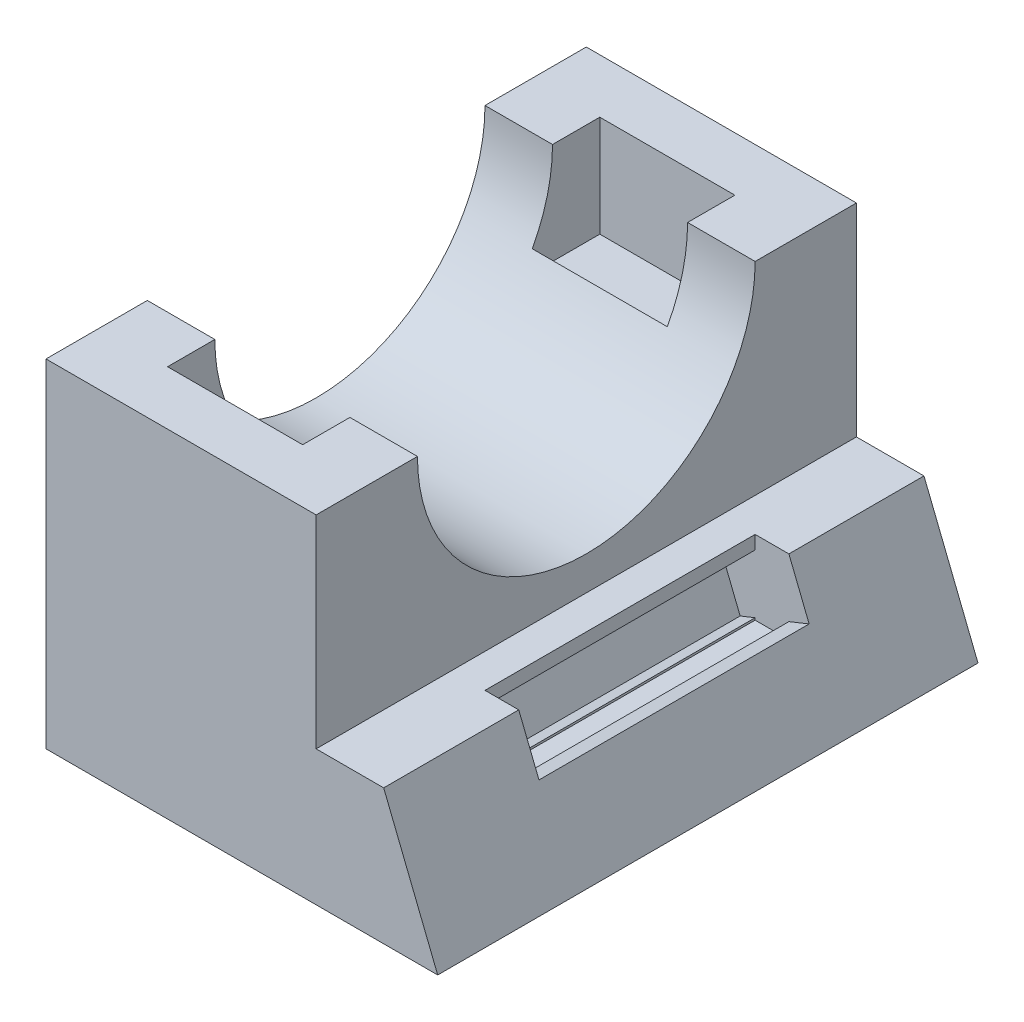
ISO-10303-21;
HEADER;
FILE_DESCRIPTION(('STEP AP214'),'2;1');
FILE_NAME('part.step','',(''),(''),'','','');
FILE_SCHEMA(('AUTOMOTIVE_DESIGN { 1 0 10303 214 1 1 1 1 }'));
ENDSEC;
DATA;
#1=APPLICATION_CONTEXT('core data for automotive mechanical design processes');
#2=APPLICATION_PROTOCOL_DEFINITION('international standard','automotive_design',2000,#1);
#3=PRODUCT_CONTEXT('',#1,'mechanical');
#4=PRODUCT('Part','Part','',(#3));
#5=PRODUCT_RELATED_PRODUCT_CATEGORY('part','',(#4));
#6=PRODUCT_DEFINITION_FORMATION('','',#4);
#7=PRODUCT_DEFINITION_CONTEXT('part definition',#1,'design');
#8=PRODUCT_DEFINITION('design','',#6,#7);
#9=PRODUCT_DEFINITION_SHAPE('','',#8);
#10=(LENGTH_UNIT() NAMED_UNIT(*) SI_UNIT(.MILLI.,.METRE.));
#11=(NAMED_UNIT(*) PLANE_ANGLE_UNIT() SI_UNIT($,.RADIAN.));
#12=(NAMED_UNIT(*) SI_UNIT($,.STERADIAN.) SOLID_ANGLE_UNIT());
#13=UNCERTAINTY_MEASURE_WITH_UNIT(LENGTH_MEASURE(1.E-05),#10,'distance_accuracy_value','');
#14=(GEOMETRIC_REPRESENTATION_CONTEXT(3) GLOBAL_UNCERTAINTY_ASSIGNED_CONTEXT((#13)) GLOBAL_UNIT_ASSIGNED_CONTEXT((#10,
#11,#12)) REPRESENTATION_CONTEXT('',''));
#15=CARTESIAN_POINT('',(0.,0.,0.));
#16=DIRECTION('',(0.,0.,1.));
#17=DIRECTION('',(1.,0.,0.));
#18=AXIS2_PLACEMENT_3D('',#15,#16,#17);
#19=CARTESIAN_POINT('',(45.,9.00000000000001,20.));
#20=DIRECTION('',(-1.,0.,0.));
#21=DIRECTION('',(0.,0.,1.));
#22=AXIS2_PLACEMENT_3D('',#19,#20,#21);
#23=PLANE('',#22);
#24=DIRECTION('',(0.,1.,0.));
#25=VECTOR('',#24,1.);
#26=CARTESIAN_POINT('',(45.,9.00000000000001,60.));
#27=LINE('',#26,#25);
#28=CARTESIAN_POINT('',(45.,18.,60.));
#29=VERTEX_POINT('',#28);
#30=CARTESIAN_POINT('',(45.,20.,60.));
#31=VERTEX_POINT('',#30);
#32=EDGE_CURVE('E297',#29,#31,#27,.T.);
#33=ORIENTED_EDGE('',*,*,#32,.F.);
#34=DIRECTION('',(0.,0.,-1.));
#35=VECTOR('',#34,1.);
#36=CARTESIAN_POINT('',(45.,18.,20.));
#37=LINE('',#36,#35);
#38=CARTESIAN_POINT('',(45.,18.,20.));
#39=VERTEX_POINT('',#38);
#40=EDGE_CURVE('E229',#29,#39,#37,.T.);
#41=ORIENTED_EDGE('',*,*,#40,.T.);
#42=DIRECTION('',(0.,1.,0.));
#43=VECTOR('',#42,1.);
#44=CARTESIAN_POINT('',(45.,9.00000000000001,20.));
#45=LINE('',#44,#43);
#46=CARTESIAN_POINT('',(45.,20.,20.));
#47=VERTEX_POINT('',#46);
#48=EDGE_CURVE('E298',#39,#47,#45,.T.);
#49=ORIENTED_EDGE('',*,*,#48,.T.);
#50=DIRECTION('',(0.,0.,1.));
#51=VECTOR('',#50,1.);
#52=CARTESIAN_POINT('',(45.,20.,20.));
#53=LINE('',#52,#51);
#54=EDGE_CURVE('E283',#47,#31,#53,.T.);
#55=ORIENTED_EDGE('',*,*,#54,.T.);
#56=EDGE_LOOP('',(#33,#41,#49,#55));
#57=FACE_BOUND('',#56,.T.);
#58=ADVANCED_FACE('F39',(#57),#23,.F.);
#59=CARTESIAN_POINT('',(0.,50.,80.));
#60=DIRECTION('',(0.,-1.,0.));
#61=DIRECTION('',(0.,0.,-1.));
#62=AXIS2_PLACEMENT_3D('',#59,#60,#61);
#63=PLANE('',#62);
#64=DIRECTION('',(0.,0.,-1.));
#65=VECTOR('',#64,1.);
#66=CARTESIAN_POINT('',(0.,50.,80.));
#67=LINE('',#66,#65);
#68=CARTESIAN_POINT('',(0.,50.,15.));
#69=VERTEX_POINT('',#68);
#70=CARTESIAN_POINT('',(0.,50.,0.));
#71=VERTEX_POINT('',#70);
#72=EDGE_CURVE('E428',#69,#71,#67,.T.);
#73=ORIENTED_EDGE('',*,*,#72,.F.);
#74=DIRECTION('',(1.,0.,0.));
#75=VECTOR('',#74,1.);
#76=CARTESIAN_POINT('',(0.,50.,15.));
#77=LINE('',#76,#75);
#78=CARTESIAN_POINT('',(10.,50.,15.));
#79=VERTEX_POINT('',#78);
#80=EDGE_CURVE('E323',#69,#79,#77,.T.);
#81=ORIENTED_EDGE('',*,*,#80,.T.);
#82=DIRECTION('',(0.,0.,1.));
#83=VECTOR('',#82,1.);
#84=CARTESIAN_POINT('',(10.,50.,18.));
#85=LINE('',#84,#83);
#86=CARTESIAN_POINT('',(10.,50.,8.00000000000001));
#87=VERTEX_POINT('',#86);
#88=EDGE_CURVE('E341',#87,#79,#85,.T.);
#89=ORIENTED_EDGE('',*,*,#88,.F.);
#90=DIRECTION('',(-1.,0.,0.));
#91=VECTOR('',#90,1.);
#92=CARTESIAN_POINT('',(10.,50.,8.00000000000001));
#93=LINE('',#92,#91);
#94=CARTESIAN_POINT('',(30.,50.,8.00000000000001));
#95=VERTEX_POINT('',#94);
#96=EDGE_CURVE('E353',#95,#87,#93,.T.);
#97=ORIENTED_EDGE('',*,*,#96,.F.);
#98=DIRECTION('',(0.,0.,-1.));
#99=VECTOR('',#98,1.);
#100=CARTESIAN_POINT('',(30.,50.,8.00000000000001));
#101=LINE('',#100,#99);
#102=CARTESIAN_POINT('',(30.,50.,15.));
#103=VERTEX_POINT('',#102);
#104=EDGE_CURVE('E355',#103,#95,#101,.T.);
#105=ORIENTED_EDGE('',*,*,#104,.F.);
#106=CARTESIAN_POINT('',(40.,50.,15.));
#107=VERTEX_POINT('',#106);
#108=EDGE_CURVE('E317',#103,#107,#77,.T.);
#109=ORIENTED_EDGE('',*,*,#108,.T.);
#110=DIRECTION('',(0.,0.,-1.));
#111=VECTOR('',#110,1.);
#112=CARTESIAN_POINT('',(40.,50.,80.));
#113=LINE('',#112,#111);
#114=CARTESIAN_POINT('',(40.,50.,0.));
#115=VERTEX_POINT('',#114);
#116=EDGE_CURVE('E435',#107,#115,#113,.T.);
#117=ORIENTED_EDGE('',*,*,#116,.T.);
#118=DIRECTION('',(-1.,0.,0.));
#119=VECTOR('',#118,1.);
#120=CARTESIAN_POINT('',(0.,50.,0.));
#121=LINE('',#120,#119);
#122=EDGE_CURVE('E425',#115,#71,#121,.T.);
#123=ORIENTED_EDGE('',*,*,#122,.T.);
#124=EDGE_LOOP('',(#73,#81,#89,#97,#105,#109,#117,#123));
#125=FACE_BOUND('',#124,.T.);
#126=ADVANCED_FACE('F456',(#125),#63,.F.);
#127=CARTESIAN_POINT('',(58.,0.,80.));
#128=DIRECTION('',(0.,1.,0.));
#129=DIRECTION('',(0.,0.,1.));
#130=AXIS2_PLACEMENT_3D('',#127,#128,#129);
#131=PLANE('',#130);
#132=DIRECTION('',(1.,0.,0.));
#133=VECTOR('',#132,1.);
#134=CARTESIAN_POINT('',(58.,0.,0.));
#135=LINE('',#134,#133);
#136=CARTESIAN_POINT('',(0.,0.,0.));
#137=VERTEX_POINT('',#136);
#138=CARTESIAN_POINT('',(58.,0.,0.));
#139=VERTEX_POINT('',#138);
#140=EDGE_CURVE('E365',#137,#139,#135,.T.);
#141=ORIENTED_EDGE('',*,*,#140,.T.);
#142=DIRECTION('',(0.,0.,-1.));
#143=VECTOR('',#142,1.);
#144=CARTESIAN_POINT('',(58.,0.,80.));
#145=LINE('',#144,#143);
#146=CARTESIAN_POINT('',(58.,0.,80.));
#147=VERTEX_POINT('',#146);
#148=EDGE_CURVE('E50',#147,#139,#145,.T.);
#149=ORIENTED_EDGE('',*,*,#148,.F.);
#150=DIRECTION('',(1.,0.,0.));
#151=VECTOR('',#150,1.);
#152=CARTESIAN_POINT('',(58.,0.,80.));
#153=LINE('',#152,#151);
#154=CARTESIAN_POINT('',(0.,0.,80.));
#155=VERTEX_POINT('',#154);
#156=EDGE_CURVE('E405',#155,#147,#153,.T.);
#157=ORIENTED_EDGE('',*,*,#156,.F.);
#158=DIRECTION('',(0.,0.,-1.));
#159=VECTOR('',#158,1.);
#160=CARTESIAN_POINT('',(0.,0.,80.));
#161=LINE('',#160,#159);
#162=EDGE_CURVE('E414',#155,#137,#161,.T.);
#163=ORIENTED_EDGE('',*,*,#162,.T.);
#164=EDGE_LOOP('',(#141,#149,#157,#163));
#165=FACE_BOUND('',#164,.T.);
#166=ADVANCED_FACE('F41',(#165),#131,.F.);
#167=CARTESIAN_POINT('',(40.,20.,80.));
#168=DIRECTION('',(0.,-1.,0.));
#169=DIRECTION('',(0.,0.,-1.));
#170=AXIS2_PLACEMENT_3D('',#167,#168,#169);
#171=PLANE('',#170);
#172=DIRECTION('',(0.,0.,1.));
#173=VECTOR('',#172,1.);
#174=CARTESIAN_POINT('',(50.,20.,0.));
#175=LINE('',#174,#173);
#176=CARTESIAN_POINT('',(50.,20.,60.));
#177=VERTEX_POINT('',#176);
#178=CARTESIAN_POINT('',(50.,20.,80.));
#179=VERTEX_POINT('',#178);
#180=EDGE_CURVE('E308',#177,#179,#175,.T.);
#181=ORIENTED_EDGE('',*,*,#180,.F.);
#182=DIRECTION('',(1.,0.,0.));
#183=VECTOR('',#182,1.);
#184=CARTESIAN_POINT('',(45.,20.,60.));
#185=LINE('',#184,#183);
#186=EDGE_CURVE('E272',#31,#177,#185,.T.);
#187=ORIENTED_EDGE('',*,*,#186,.F.);
#188=ORIENTED_EDGE('',*,*,#54,.F.);
#189=DIRECTION('',(-1.,0.,0.));
#190=VECTOR('',#189,1.);
#191=CARTESIAN_POINT('',(50.,20.,20.));
#192=LINE('',#191,#190);
#193=CARTESIAN_POINT('',(50.,20.,20.));
#194=VERTEX_POINT('',#193);
#195=EDGE_CURVE('E268',#194,#47,#192,.T.);
#196=ORIENTED_EDGE('',*,*,#195,.F.);
#197=CARTESIAN_POINT('',(50.,20.,0.));
#198=VERTEX_POINT('',#197);
#199=EDGE_CURVE('E306',#198,#194,#175,.T.);
#200=ORIENTED_EDGE('',*,*,#199,.F.);
#201=DIRECTION('',(-1.,0.,0.));
#202=VECTOR('',#201,1.);
#203=CARTESIAN_POINT('',(40.,20.,0.));
#204=LINE('',#203,#202);
#205=CARTESIAN_POINT('',(40.,20.,0.));
#206=VERTEX_POINT('',#205);
#207=EDGE_CURVE('E417',#198,#206,#204,.T.);
#208=ORIENTED_EDGE('',*,*,#207,.T.);
#209=DIRECTION('',(0.,0.,-1.));
#210=VECTOR('',#209,1.);
#211=CARTESIAN_POINT('',(40.,20.,80.));
#212=LINE('',#211,#210);
#213=CARTESIAN_POINT('',(40.,20.,80.));
#214=VERTEX_POINT('',#213);
#215=EDGE_CURVE('E436',#214,#206,#212,.T.);
#216=ORIENTED_EDGE('',*,*,#215,.F.);
#217=DIRECTION('',(-1.,0.,0.));
#218=VECTOR('',#217,1.);
#219=CARTESIAN_POINT('',(40.,20.,80.));
#220=LINE('',#219,#218);
#221=EDGE_CURVE('E403',#179,#214,#220,.T.);
#222=ORIENTED_EDGE('',*,*,#221,.F.);
#223=EDGE_LOOP('',(#181,#187,#188,#196,#200,#208,#216,#222));
#224=FACE_BOUND('',#223,.T.);
#225=ADVANCED_FACE('F473',(#224),#171,.F.);
#226=CARTESIAN_POINT('',(40.,50.,80.));
#227=DIRECTION('',(-1.,0.,0.));
#228=DIRECTION('',(0.,-1.,0.));
#229=AXIS2_PLACEMENT_3D('',#226,#227,#228);
#230=PLANE('',#229);
#231=ORIENTED_EDGE('',*,*,#116,.F.);
#232=CARTESIAN_POINT('',(40.,50.,40.));
#233=DIRECTION('',(1.,0.,0.));
#234=DIRECTION('',(0.,1.,0.));
#235=AXIS2_PLACEMENT_3D('',#232,#233,#234);
#236=CIRCLE('',#235,25.);
#237=CARTESIAN_POINT('',(40.,50.,65.));
#238=VERTEX_POINT('',#237);
#239=EDGE_CURVE('E313',#238,#107,#236,.T.);
#240=ORIENTED_EDGE('',*,*,#239,.F.);
#241=CARTESIAN_POINT('',(40.,50.,80.));
#242=VERTEX_POINT('',#241);
#243=EDGE_CURVE('E433',#242,#238,#113,.T.);
#244=ORIENTED_EDGE('',*,*,#243,.F.);
#245=DIRECTION('',(0.,1.,0.));
#246=VECTOR('',#245,1.);
#247=CARTESIAN_POINT('',(40.,50.,80.));
#248=LINE('',#247,#246);
#249=EDGE_CURVE('E410',#214,#242,#248,.T.);
#250=ORIENTED_EDGE('',*,*,#249,.F.);
#251=ORIENTED_EDGE('',*,*,#215,.T.);
#252=DIRECTION('',(0.,1.,0.));
#253=VECTOR('',#252,1.);
#254=CARTESIAN_POINT('',(40.,50.,0.));
#255=LINE('',#254,#253);
#256=EDGE_CURVE('E420',#206,#115,#255,.T.);
#257=ORIENTED_EDGE('',*,*,#256,.T.);
#258=EDGE_LOOP('',(#231,#240,#244,#250,#251,#257));
#259=FACE_BOUND('',#258,.T.);
#260=ADVANCED_FACE('F461',(#259),#230,.F.);
#261=ORIENTED_EDGE('',*,*,#243,.T.);
#262=DIRECTION('',(1.,0.,0.));
#263=VECTOR('',#262,1.);
#264=CARTESIAN_POINT('',(0.,50.,65.));
#265=LINE('',#264,#263);
#266=CARTESIAN_POINT('',(30.,50.,65.));
#267=VERTEX_POINT('',#266);
#268=EDGE_CURVE('E337',#238,#267,#265,.F.);
#269=ORIENTED_EDGE('',*,*,#268,.T.);
#270=DIRECTION('',(0.,0.,-1.));
#271=VECTOR('',#270,1.);
#272=CARTESIAN_POINT('',(30.,50.,72.));
#273=LINE('',#272,#271);
#274=CARTESIAN_POINT('',(30.,50.,72.));
#275=VERTEX_POINT('',#274);
#276=EDGE_CURVE('E376',#275,#267,#273,.T.);
#277=ORIENTED_EDGE('',*,*,#276,.F.);
#278=DIRECTION('',(1.,0.,0.));
#279=VECTOR('',#278,1.);
#280=CARTESIAN_POINT('',(10.,50.,72.));
#281=LINE('',#280,#279);
#282=CARTESIAN_POINT('',(10.,50.,72.));
#283=VERTEX_POINT('',#282);
#284=EDGE_CURVE('E389',#283,#275,#281,.T.);
#285=ORIENTED_EDGE('',*,*,#284,.F.);
#286=DIRECTION('',(0.,0.,1.));
#287=VECTOR('',#286,1.);
#288=CARTESIAN_POINT('',(10.,50.,62.));
#289=LINE('',#288,#287);
#290=CARTESIAN_POINT('',(10.,50.,65.));
#291=VERTEX_POINT('',#290);
#292=EDGE_CURVE('E387',#291,#283,#289,.T.);
#293=ORIENTED_EDGE('',*,*,#292,.F.);
#294=CARTESIAN_POINT('',(0.,50.,65.));
#295=VERTEX_POINT('',#294);
#296=EDGE_CURVE('E335',#291,#295,#265,.F.);
#297=ORIENTED_EDGE('',*,*,#296,.T.);
#298=CARTESIAN_POINT('',(0.,50.,80.));
#299=VERTEX_POINT('',#298);
#300=EDGE_CURVE('E427',#299,#295,#67,.T.);
#301=ORIENTED_EDGE('',*,*,#300,.F.);
#302=DIRECTION('',(-1.,0.,0.));
#303=VECTOR('',#302,1.);
#304=CARTESIAN_POINT('',(0.,50.,80.));
#305=LINE('',#304,#303);
#306=EDGE_CURVE('E408',#242,#299,#305,.T.);
#307=ORIENTED_EDGE('',*,*,#306,.F.);
#308=EDGE_LOOP('',(#261,#269,#277,#285,#293,#297,#301,#307));
#309=FACE_BOUND('',#308,.T.);
#310=ADVANCED_FACE('F488',(#309),#63,.F.);
#311=CARTESIAN_POINT('',(0.,0.,80.));
#312=DIRECTION('',(1.,0.,0.));
#313=DIRECTION('',(0.,0.,-1.));
#314=AXIS2_PLACEMENT_3D('',#311,#312,#313);
#315=PLANE('',#314);
#316=ORIENTED_EDGE('',*,*,#300,.T.);
#317=CARTESIAN_POINT('',(0.,50.,40.));
#318=DIRECTION('',(1.,0.,0.));
#319=DIRECTION('',(0.,1.,0.));
#320=AXIS2_PLACEMENT_3D('',#317,#318,#319);
#321=CIRCLE('',#320,25.);
#322=EDGE_CURVE('E315',#295,#69,#321,.T.);
#323=ORIENTED_EDGE('',*,*,#322,.T.);
#324=ORIENTED_EDGE('',*,*,#72,.T.);
#325=DIRECTION('',(0.,-1.,0.));
#326=VECTOR('',#325,1.);
#327=CARTESIAN_POINT('',(0.,0.,0.));
#328=LINE('',#327,#326);
#329=EDGE_CURVE('E407',#71,#137,#328,.T.);
#330=ORIENTED_EDGE('',*,*,#329,.T.);
#331=ORIENTED_EDGE('',*,*,#162,.F.);
#332=DIRECTION('',(0.,-1.,0.));
#333=VECTOR('',#332,1.);
#334=CARTESIAN_POINT('',(0.,0.,80.));
#335=LINE('',#334,#333);
#336=EDGE_CURVE('E415',#299,#155,#335,.T.);
#337=ORIENTED_EDGE('',*,*,#336,.F.);
#338=EDGE_LOOP('',(#316,#323,#324,#330,#331,#337));
#339=FACE_BOUND('',#338,.T.);
#340=ADVANCED_FACE('F454',(#339),#315,.F.);
#341=CARTESIAN_POINT('',(0.,0.,80.));
#342=DIRECTION('',(0.,0.,-1.));
#343=DIRECTION('',(-1.,0.,0.));
#344=AXIS2_PLACEMENT_3D('',#341,#342,#343);
#345=PLANE('',#344);
#346=ORIENTED_EDGE('',*,*,#156,.T.);
#347=DIRECTION('',(0.371390676354104,-0.928476690885259,0.));
#348=VECTOR('',#347,1.);
#349=CARTESIAN_POINT('',(58.,0.,80.));
#350=LINE('',#349,#348);
#351=EDGE_CURVE('E291',#179,#147,#350,.T.);
#352=ORIENTED_EDGE('',*,*,#351,.F.);
#353=ORIENTED_EDGE('',*,*,#221,.T.);
#354=ORIENTED_EDGE('',*,*,#249,.T.);
#355=ORIENTED_EDGE('',*,*,#306,.T.);
#356=ORIENTED_EDGE('',*,*,#336,.T.);
#357=EDGE_LOOP('',(#346,#352,#353,#354,#355,#356));
#358=FACE_BOUND('',#357,.T.);
#359=ADVANCED_FACE('F482',(#358),#345,.F.);
#360=CARTESIAN_POINT('',(0.,0.,0.));
#361=DIRECTION('',(0.,0.,-1.));
#362=DIRECTION('',(-1.,0.,0.));
#363=AXIS2_PLACEMENT_3D('',#360,#361,#362);
#364=PLANE('',#363);
#365=DIRECTION('',(0.371390676354104,-0.928476690885259,0.));
#366=VECTOR('',#365,1.);
#367=CARTESIAN_POINT('',(58.,0.,0.));
#368=LINE('',#367,#366);
#369=EDGE_CURVE('E301',#198,#139,#368,.T.);
#370=ORIENTED_EDGE('',*,*,#369,.T.);
#371=ORIENTED_EDGE('',*,*,#140,.F.);
#372=ORIENTED_EDGE('',*,*,#329,.F.);
#373=ORIENTED_EDGE('',*,*,#122,.F.);
#374=ORIENTED_EDGE('',*,*,#256,.F.);
#375=ORIENTED_EDGE('',*,*,#207,.F.);
#376=EDGE_LOOP('',(#370,#371,#372,#373,#374,#375));
#377=FACE_BOUND('',#376,.T.);
#378=ADVANCED_FACE('F450',(#377),#364,.T.);
#379=CARTESIAN_POINT('',(30.,35.,62.));
#380=DIRECTION('',(0.,0.,-1.));
#381=DIRECTION('',(-1.,0.,0.));
#382=AXIS2_PLACEMENT_3D('',#379,#380,#381);
#383=PLANE('',#382);
#384=DIRECTION('',(0.,1.,0.));
#385=VECTOR('',#384,1.);
#386=CARTESIAN_POINT('',(30.,35.,62.));
#387=LINE('',#386,#385);
#388=CARTESIAN_POINT('',(30.,35.,62.));
#389=VERTEX_POINT('',#388);
#390=CARTESIAN_POINT('',(30.,38.1256579129621,62.));
#391=VERTEX_POINT('',#390);
#392=EDGE_CURVE('E358',#389,#391,#387,.T.);
#393=ORIENTED_EDGE('',*,*,#392,.T.);
#394=DIRECTION('',(1.,0.,0.));
#395=VECTOR('',#394,1.);
#396=CARTESIAN_POINT('',(0.,38.1256579129621,62.));
#397=LINE('',#396,#395);
#398=CARTESIAN_POINT('',(10.,38.1256579129621,62.));
#399=VERTEX_POINT('',#398);
#400=EDGE_CURVE('E328',#391,#399,#397,.F.);
#401=ORIENTED_EDGE('',*,*,#400,.T.);
#402=DIRECTION('',(0.,1.,0.));
#403=VECTOR('',#402,1.);
#404=CARTESIAN_POINT('',(10.,35.,62.));
#405=LINE('',#404,#403);
#406=CARTESIAN_POINT('',(10.,35.,62.));
#407=VERTEX_POINT('',#406);
#408=EDGE_CURVE('E384',#407,#399,#405,.T.);
#409=ORIENTED_EDGE('',*,*,#408,.F.);
#410=DIRECTION('',(-1.,0.,0.));
#411=VECTOR('',#410,1.);
#412=CARTESIAN_POINT('',(30.,35.,62.));
#413=LINE('',#412,#411);
#414=EDGE_CURVE('E375',#389,#407,#413,.T.);
#415=ORIENTED_EDGE('',*,*,#414,.F.);
#416=EDGE_LOOP('',(#393,#401,#409,#415));
#417=FACE_BOUND('',#416,.T.);
#418=ADVANCED_FACE('F604',(#417),#383,.F.);
#419=CARTESIAN_POINT('',(30.,35.,72.));
#420=DIRECTION('',(1.,0.,0.));
#421=DIRECTION('',(0.,0.,-1.));
#422=AXIS2_PLACEMENT_3D('',#419,#420,#421);
#423=PLANE('',#422);
#424=ORIENTED_EDGE('',*,*,#276,.T.);
#425=CARTESIAN_POINT('',(30.,50.,40.));
#426=DIRECTION('',(1.,0.,0.));
#427=DIRECTION('',(0.,0.,-1.));
#428=AXIS2_PLACEMENT_3D('',#425,#426,#427);
#429=CIRCLE('',#428,25.);
#430=EDGE_CURVE('E333',#267,#391,#429,.T.);
#431=ORIENTED_EDGE('',*,*,#430,.T.);
#432=ORIENTED_EDGE('',*,*,#392,.F.);
#433=DIRECTION('',(0.,0.,-1.));
#434=VECTOR('',#433,1.);
#435=CARTESIAN_POINT('',(30.,35.,72.));
#436=LINE('',#435,#434);
#437=CARTESIAN_POINT('',(30.,35.,72.));
#438=VERTEX_POINT('',#437);
#439=EDGE_CURVE('E385',#438,#389,#436,.T.);
#440=ORIENTED_EDGE('',*,*,#439,.F.);
#441=DIRECTION('',(0.,1.,0.));
#442=VECTOR('',#441,1.);
#443=CARTESIAN_POINT('',(30.,35.,72.));
#444=LINE('',#443,#442);
#445=EDGE_CURVE('E393',#438,#275,#444,.T.);
#446=ORIENTED_EDGE('',*,*,#445,.T.);
#447=EDGE_LOOP('',(#424,#431,#432,#440,#446));
#448=FACE_BOUND('',#447,.T.);
#449=ADVANCED_FACE('F663',(#448),#423,.F.);
#450=CARTESIAN_POINT('',(10.,35.,72.));
#451=DIRECTION('',(0.,0.,1.));
#452=DIRECTION('',(1.,0.,0.));
#453=AXIS2_PLACEMENT_3D('',#450,#451,#452);
#454=PLANE('',#453);
#455=ORIENTED_EDGE('',*,*,#284,.T.);
#456=ORIENTED_EDGE('',*,*,#445,.F.);
#457=DIRECTION('',(1.,0.,0.));
#458=VECTOR('',#457,1.);
#459=CARTESIAN_POINT('',(10.,35.,72.));
#460=LINE('',#459,#458);
#461=CARTESIAN_POINT('',(10.,35.,72.));
#462=VERTEX_POINT('',#461);
#463=EDGE_CURVE('E377',#462,#438,#460,.T.);
#464=ORIENTED_EDGE('',*,*,#463,.F.);
#465=DIRECTION('',(0.,1.,0.));
#466=VECTOR('',#465,1.);
#467=CARTESIAN_POINT('',(10.,35.,72.));
#468=LINE('',#467,#466);
#469=EDGE_CURVE('E400',#462,#283,#468,.T.);
#470=ORIENTED_EDGE('',*,*,#469,.T.);
#471=EDGE_LOOP('',(#455,#456,#464,#470));
#472=FACE_BOUND('',#471,.T.);
#473=ADVANCED_FACE('F657',(#472),#454,.F.);
#474=CARTESIAN_POINT('',(10.,35.,62.));
#475=DIRECTION('',(-1.,0.,0.));
#476=DIRECTION('',(0.,0.,1.));
#477=AXIS2_PLACEMENT_3D('',#474,#475,#476);
#478=PLANE('',#477);
#479=ORIENTED_EDGE('',*,*,#408,.T.);
#480=CARTESIAN_POINT('',(9.99999999999999,50.,40.));
#481=DIRECTION('',(-1.,0.,0.));
#482=DIRECTION('',(0.,0.,1.));
#483=AXIS2_PLACEMENT_3D('',#480,#481,#482);
#484=CIRCLE('',#483,25.);
#485=EDGE_CURVE('E326',#399,#291,#484,.T.);
#486=ORIENTED_EDGE('',*,*,#485,.T.);
#487=ORIENTED_EDGE('',*,*,#292,.T.);
#488=ORIENTED_EDGE('',*,*,#469,.F.);
#489=DIRECTION('',(0.,0.,1.));
#490=VECTOR('',#489,1.);
#491=CARTESIAN_POINT('',(10.,35.,62.));
#492=LINE('',#491,#490);
#493=EDGE_CURVE('E374',#407,#462,#492,.T.);
#494=ORIENTED_EDGE('',*,*,#493,.F.);
#495=EDGE_LOOP('',(#479,#486,#487,#488,#494));
#496=FACE_BOUND('',#495,.T.);
#497=ADVANCED_FACE('F652',(#496),#478,.F.);
#498=CARTESIAN_POINT('',(0.,35.,0.));
#499=DIRECTION('',(0.,1.,0.));
#500=DIRECTION('',(0.,0.,1.));
#501=AXIS2_PLACEMENT_3D('',#498,#499,#500);
#502=PLANE('',#501);
#503=ORIENTED_EDGE('',*,*,#414,.T.);
#504=ORIENTED_EDGE('',*,*,#493,.T.);
#505=ORIENTED_EDGE('',*,*,#463,.T.);
#506=ORIENTED_EDGE('',*,*,#439,.T.);
#507=EDGE_LOOP('',(#503,#504,#505,#506));
#508=FACE_BOUND('',#507,.T.);
#509=ADVANCED_FACE('F648',(#508),#502,.T.);
#510=CARTESIAN_POINT('',(30.,35.,18.));
#511=DIRECTION('',(0.,0.,1.));
#512=DIRECTION('',(1.,0.,0.));
#513=AXIS2_PLACEMENT_3D('',#510,#511,#512);
#514=PLANE('',#513);
#515=DIRECTION('',(0.,1.,0.));
#516=VECTOR('',#515,1.);
#517=CARTESIAN_POINT('',(10.,35.,18.));
#518=LINE('',#517,#516);
#519=CARTESIAN_POINT('',(10.,35.,18.));
#520=VERTEX_POINT('',#519);
#521=CARTESIAN_POINT('',(10.,38.1256579129621,18.));
#522=VERTEX_POINT('',#521);
#523=EDGE_CURVE('E363',#520,#522,#518,.T.);
#524=ORIENTED_EDGE('',*,*,#523,.T.);
#525=DIRECTION('',(1.,0.,0.));
#526=VECTOR('',#525,1.);
#527=CARTESIAN_POINT('',(0.,38.125657912962,18.));
#528=LINE('',#527,#526);
#529=CARTESIAN_POINT('',(30.,38.1256579129621,18.));
#530=VERTEX_POINT('',#529);
#531=EDGE_CURVE('E312',#522,#530,#528,.T.);
#532=ORIENTED_EDGE('',*,*,#531,.T.);
#533=DIRECTION('',(0.,1.,0.));
#534=VECTOR('',#533,1.);
#535=CARTESIAN_POINT('',(30.,35.,18.));
#536=LINE('',#535,#534);
#537=CARTESIAN_POINT('',(30.,35.,18.));
#538=VERTEX_POINT('',#537);
#539=EDGE_CURVE('E354',#538,#530,#536,.T.);
#540=ORIENTED_EDGE('',*,*,#539,.F.);
#541=DIRECTION('',(1.,0.,0.));
#542=VECTOR('',#541,1.);
#543=CARTESIAN_POINT('',(30.,35.,18.));
#544=LINE('',#543,#542);
#545=EDGE_CURVE('E336',#520,#538,#544,.T.);
#546=ORIENTED_EDGE('',*,*,#545,.F.);
#547=EDGE_LOOP('',(#524,#532,#540,#546));
#548=FACE_BOUND('',#547,.T.);
#549=ADVANCED_FACE('F501',(#548),#514,.F.);
#550=CARTESIAN_POINT('',(10.,35.,18.));
#551=DIRECTION('',(-1.,0.,0.));
#552=DIRECTION('',(0.,0.,1.));
#553=AXIS2_PLACEMENT_3D('',#550,#551,#552);
#554=PLANE('',#553);
#555=ORIENTED_EDGE('',*,*,#88,.T.);
#556=CARTESIAN_POINT('',(10.,50.,40.));
#557=DIRECTION('',(-1.,0.,0.));
#558=DIRECTION('',(0.,0.,1.));
#559=AXIS2_PLACEMENT_3D('',#556,#557,#558);
#560=CIRCLE('',#559,25.);
#561=EDGE_CURVE('E325',#79,#522,#560,.T.);
#562=ORIENTED_EDGE('',*,*,#561,.T.);
#563=ORIENTED_EDGE('',*,*,#523,.F.);
#564=DIRECTION('',(0.,0.,1.));
#565=VECTOR('',#564,1.);
#566=CARTESIAN_POINT('',(10.,35.,18.));
#567=LINE('',#566,#565);
#568=CARTESIAN_POINT('',(10.,35.,8.00000000000001));
#569=VERTEX_POINT('',#568);
#570=EDGE_CURVE('E349',#569,#520,#567,.T.);
#571=ORIENTED_EDGE('',*,*,#570,.F.);
#572=DIRECTION('',(0.,1.,0.));
#573=VECTOR('',#572,1.);
#574=CARTESIAN_POINT('',(10.,35.,8.00000000000001));
#575=LINE('',#574,#573);
#576=EDGE_CURVE('E364',#569,#87,#575,.T.);
#577=ORIENTED_EDGE('',*,*,#576,.T.);
#578=EDGE_LOOP('',(#555,#562,#563,#571,#577));
#579=FACE_BOUND('',#578,.T.);
#580=ADVANCED_FACE('F494',(#579),#554,.F.);
#581=CARTESIAN_POINT('',(10.,35.,8.00000000000001));
#582=DIRECTION('',(0.,0.,-1.));
#583=DIRECTION('',(-1.,0.,0.));
#584=AXIS2_PLACEMENT_3D('',#581,#582,#583);
#585=PLANE('',#584);
#586=ORIENTED_EDGE('',*,*,#96,.T.);
#587=ORIENTED_EDGE('',*,*,#576,.F.);
#588=DIRECTION('',(-1.,0.,0.));
#589=VECTOR('',#588,1.);
#590=CARTESIAN_POINT('',(10.,35.,8.00000000000001));
#591=LINE('',#590,#589);
#592=CARTESIAN_POINT('',(30.,35.,8.00000000000001));
#593=VERTEX_POINT('',#592);
#594=EDGE_CURVE('E347',#593,#569,#591,.T.);
#595=ORIENTED_EDGE('',*,*,#594,.F.);
#596=DIRECTION('',(0.,1.,0.));
#597=VECTOR('',#596,1.);
#598=CARTESIAN_POINT('',(30.,35.,8.00000000000001));
#599=LINE('',#598,#597);
#600=EDGE_CURVE('E370',#593,#95,#599,.T.);
#601=ORIENTED_EDGE('',*,*,#600,.T.);
#602=EDGE_LOOP('',(#586,#587,#595,#601));
#603=FACE_BOUND('',#602,.T.);
#604=ADVANCED_FACE('F496',(#603),#585,.F.);
#605=CARTESIAN_POINT('',(30.,35.,8.00000000000001));
#606=DIRECTION('',(1.,0.,0.));
#607=DIRECTION('',(0.,0.,-1.));
#608=AXIS2_PLACEMENT_3D('',#605,#606,#607);
#609=PLANE('',#608);
#610=ORIENTED_EDGE('',*,*,#539,.T.);
#611=CARTESIAN_POINT('',(30.,50.,40.));
#612=DIRECTION('',(1.,0.,0.));
#613=DIRECTION('',(0.,0.,-1.));
#614=AXIS2_PLACEMENT_3D('',#611,#612,#613);
#615=CIRCLE('',#614,25.);
#616=EDGE_CURVE('E11',#530,#103,#615,.T.);
#617=ORIENTED_EDGE('',*,*,#616,.T.);
#618=ORIENTED_EDGE('',*,*,#104,.T.);
#619=ORIENTED_EDGE('',*,*,#600,.F.);
#620=DIRECTION('',(0.,0.,-1.));
#621=VECTOR('',#620,1.);
#622=CARTESIAN_POINT('',(30.,35.,8.00000000000001));
#623=LINE('',#622,#621);
#624=EDGE_CURVE('E345',#538,#593,#623,.T.);
#625=ORIENTED_EDGE('',*,*,#624,.F.);
#626=EDGE_LOOP('',(#610,#617,#618,#619,#625));
#627=FACE_BOUND('',#626,.T.);
#628=ADVANCED_FACE('F502',(#627),#609,.F.);
#629=CARTESIAN_POINT('',(0.,35.,0.));
#630=DIRECTION('',(0.,-1.,0.));
#631=DIRECTION('',(0.,0.,-1.));
#632=AXIS2_PLACEMENT_3D('',#629,#630,#631);
#633=PLANE('',#632);
#634=ORIENTED_EDGE('',*,*,#545,.T.);
#635=ORIENTED_EDGE('',*,*,#624,.T.);
#636=ORIENTED_EDGE('',*,*,#594,.T.);
#637=ORIENTED_EDGE('',*,*,#570,.T.);
#638=EDGE_LOOP('',(#634,#635,#636,#637));
#639=FACE_BOUND('',#638,.T.);
#640=ADVANCED_FACE('F510',(#639),#633,.F.);
#641=CARTESIAN_POINT('',(0.,50.,40.));
#642=DIRECTION('',(1.,0.,0.));
#643=DIRECTION('',(0.,1.,0.));
#644=AXIS2_PLACEMENT_3D('',#641,#642,#643);
#645=CYLINDRICAL_SURFACE('',#644,25.);
#646=ORIENTED_EDGE('',*,*,#239,.T.);
#647=ORIENTED_EDGE('',*,*,#108,.F.);
#648=ORIENTED_EDGE('',*,*,#616,.F.);
#649=ORIENTED_EDGE('',*,*,#531,.F.);
#650=ORIENTED_EDGE('',*,*,#561,.F.);
#651=ORIENTED_EDGE('',*,*,#80,.F.);
#652=ORIENTED_EDGE('',*,*,#322,.F.);
#653=ORIENTED_EDGE('',*,*,#296,.F.);
#654=ORIENTED_EDGE('',*,*,#485,.F.);
#655=ORIENTED_EDGE('',*,*,#400,.F.);
#656=ORIENTED_EDGE('',*,*,#430,.F.);
#657=ORIENTED_EDGE('',*,*,#268,.F.);
#658=EDGE_LOOP('',(#646,#647,#648,#649,#650,#651,#652,#653,#654,#655,#656,#657));
#659=FACE_BOUND('',#658,.T.);
#660=ADVANCED_FACE('F491',(#659),#645,.F.);
#661=CARTESIAN_POINT('',(58.,0.,0.));
#662=DIRECTION('',(-0.928476690885259,-0.371390676354104,0.));
#663=DIRECTION('',(0.371390676354104,-0.928476690885259,0.));
#664=AXIS2_PLACEMENT_3D('',#661,#662,#663);
#665=PLANE('',#664);
#666=ORIENTED_EDGE('',*,*,#199,.T.);
#667=DIRECTION('',(-0.371390676354104,0.928476690885259,0.));
#668=VECTOR('',#667,1.);
#669=CARTESIAN_POINT('',(52.9950077920088,12.512480519978,20.));
#670=LINE('',#669,#668);
#671=CARTESIAN_POINT('',(52.9950077920088,12.512480519978,20.));
#672=VERTEX_POINT('',#671);
#673=EDGE_CURVE('E245',#672,#194,#670,.T.);
#674=ORIENTED_EDGE('',*,*,#673,.F.);
#675=DIRECTION('',(0.,0.,-1.));
#676=VECTOR('',#675,1.);
#677=CARTESIAN_POINT('',(52.9950077920088,12.512480519978,60.));
#678=LINE('',#677,#676);
#679=CARTESIAN_POINT('',(52.9950077920088,12.512480519978,60.));
#680=VERTEX_POINT('',#679);
#681=EDGE_CURVE('E243',#680,#672,#678,.T.);
#682=ORIENTED_EDGE('',*,*,#681,.F.);
#683=DIRECTION('',(0.371390676354104,-0.928476690885259,0.));
#684=VECTOR('',#683,1.);
#685=CARTESIAN_POINT('',(50.,20.,60.));
#686=LINE('',#685,#684);
#687=EDGE_CURVE('E247',#177,#680,#686,.T.);
#688=ORIENTED_EDGE('',*,*,#687,.F.);
#689=ORIENTED_EDGE('',*,*,#180,.T.);
#690=ORIENTED_EDGE('',*,*,#351,.T.);
#691=ORIENTED_EDGE('',*,*,#148,.T.);
#692=ORIENTED_EDGE('',*,*,#369,.F.);
#693=EDGE_LOOP('',(#666,#674,#682,#688,#689,#690,#691,#692));
#694=FACE_BOUND('',#693,.T.);
#695=ADVANCED_FACE('F439',(#694),#665,.F.);
#696=CARTESIAN_POINT('',(50.,9.00000000000001,60.));
#697=DIRECTION('',(1.,0.,0.));
#698=DIRECTION('',(0.,0.,-1.));
#699=AXIS2_PLACEMENT_3D('',#696,#697,#698);
#700=PLANE('',#699);
#701=DIRECTION('',(0.,1.,0.));
#702=VECTOR('',#701,1.);
#703=CARTESIAN_POINT('',(50.,9.00000000000001,60.));
#704=LINE('',#703,#702);
#705=CARTESIAN_POINT('',(50.,9.00000000000001,60.));
#706=VERTEX_POINT('',#705);
#707=CARTESIAN_POINT('',(50.,11.3144774031745,60.));
#708=VERTEX_POINT('',#707);
#709=EDGE_CURVE('E287',#706,#708,#704,.T.);
#710=ORIENTED_EDGE('',*,*,#709,.T.);
#711=DIRECTION('',(0.,0.,-1.));
#712=VECTOR('',#711,1.);
#713=CARTESIAN_POINT('',(50.,11.3144774031745,60.));
#714=LINE('',#713,#712);
#715=CARTESIAN_POINT('',(50.,11.3144774031745,20.));
#716=VERTEX_POINT('',#715);
#717=EDGE_CURVE('E262',#708,#716,#714,.T.);
#718=ORIENTED_EDGE('',*,*,#717,.T.);
#719=DIRECTION('',(0.,1.,0.));
#720=VECTOR('',#719,1.);
#721=CARTESIAN_POINT('',(50.,9.00000000000001,20.));
#722=LINE('',#721,#720);
#723=CARTESIAN_POINT('',(50.,9.00000000000001,20.));
#724=VERTEX_POINT('',#723);
#725=EDGE_CURVE('E284',#724,#716,#722,.T.);
#726=ORIENTED_EDGE('',*,*,#725,.F.);
#727=DIRECTION('',(0.,0.,-1.));
#728=VECTOR('',#727,1.);
#729=CARTESIAN_POINT('',(50.,9.00000000000001,60.));
#730=LINE('',#729,#728);
#731=EDGE_CURVE('E267',#706,#724,#730,.T.);
#732=ORIENTED_EDGE('',*,*,#731,.F.);
#733=EDGE_LOOP('',(#710,#718,#726,#732));
#734=FACE_BOUND('',#733,.T.);
#735=ADVANCED_FACE('F540',(#734),#700,.F.);
#736=CARTESIAN_POINT('',(45.,9.00000000000001,60.));
#737=DIRECTION('',(0.,0.,1.));
#738=DIRECTION('',(1.,0.,0.));
#739=AXIS2_PLACEMENT_3D('',#736,#737,#738);
#740=PLANE('',#739);
#741=CARTESIAN_POINT('',(45.,9.00000000000001,60.));
#742=VERTEX_POINT('',#741);
#743=CARTESIAN_POINT('',(45.,9.31447740317446,60.));
#744=VERTEX_POINT('',#743);
#745=EDGE_CURVE('E294',#742,#744,#27,.T.);
#746=ORIENTED_EDGE('',*,*,#745,.T.);
#747=DIRECTION('',(0.928476690885259,0.371390676354104,0.));
#748=VECTOR('',#747,1.);
#749=CARTESIAN_POINT('',(42.781764192271,8.42718308008285,60.));
#750=LINE('',#749,#748);
#751=CARTESIAN_POINT('',(42.781764192271,8.42718308008285,60.));
#752=VERTEX_POINT('',#751);
#753=EDGE_CURVE('E232',#752,#744,#750,.T.);
#754=ORIENTED_EDGE('',*,*,#753,.F.);
#755=DIRECTION('',(0.371390676354104,-0.928476690885259,0.));
#756=VECTOR('',#755,1.);
#757=CARTESIAN_POINT('',(39.7867564002622,15.9147025601049,60.));
#758=LINE('',#757,#756);
#759=CARTESIAN_POINT('',(39.7867564002622,15.9147025601049,60.));
#760=VERTEX_POINT('',#759);
#761=EDGE_CURVE('E235',#760,#752,#758,.T.);
#762=ORIENTED_EDGE('',*,*,#761,.F.);
#763=DIRECTION('',(0.928476690885259,0.371390676354104,0.));
#764=VECTOR('',#763,1.);
#765=CARTESIAN_POINT('',(39.7867564002622,15.9147025601049,60.));
#766=LINE('',#765,#764);
#767=EDGE_CURVE('E62',#760,#29,#766,.T.);
#768=ORIENTED_EDGE('',*,*,#767,.T.);
#769=ORIENTED_EDGE('',*,*,#32,.T.);
#770=ORIENTED_EDGE('',*,*,#186,.T.);
#771=ORIENTED_EDGE('',*,*,#687,.T.);
#772=EDGE_CURVE('E53',#708,#680,#750,.T.);
#773=ORIENTED_EDGE('',*,*,#772,.F.);
#774=ORIENTED_EDGE('',*,*,#709,.F.);
#775=DIRECTION('',(1.,0.,0.));
#776=VECTOR('',#775,1.);
#777=CARTESIAN_POINT('',(45.,9.00000000000001,60.));
#778=LINE('',#777,#776);
#779=EDGE_CURVE('E276',#742,#706,#778,.T.);
#780=ORIENTED_EDGE('',*,*,#779,.F.);
#781=EDGE_LOOP('',(#746,#754,#762,#768,#769,#770,#771,#773,#774,#780));
#782=FACE_BOUND('',#781,.T.);
#783=ADVANCED_FACE('F234',(#782),#740,.F.);
#784=CARTESIAN_POINT('',(45.,9.00000000000001,20.));
#785=VERTEX_POINT('',#784);
#786=CARTESIAN_POINT('',(45.,9.31447740317445,20.));
#787=VERTEX_POINT('',#786);
#788=EDGE_CURVE('E299',#785,#787,#45,.T.);
#789=ORIENTED_EDGE('',*,*,#788,.T.);
#790=DIRECTION('',(0.,0.,1.));
#791=VECTOR('',#790,1.);
#792=CARTESIAN_POINT('',(45.,9.31447740317445,20.));
#793=LINE('',#792,#791);
#794=EDGE_CURVE('E258',#787,#744,#793,.T.);
#795=ORIENTED_EDGE('',*,*,#794,.T.);
#796=ORIENTED_EDGE('',*,*,#745,.F.);
#797=DIRECTION('',(0.,0.,1.));
#798=VECTOR('',#797,1.);
#799=CARTESIAN_POINT('',(45.,9.00000000000001,20.));
#800=LINE('',#799,#798);
#801=EDGE_CURVE('E277',#785,#742,#800,.T.);
#802=ORIENTED_EDGE('',*,*,#801,.F.);
#803=EDGE_LOOP('',(#789,#795,#796,#802));
#804=FACE_BOUND('',#803,.T.);
#805=ADVANCED_FACE('F525',(#804),#23,.F.);
#806=CARTESIAN_POINT('',(50.,9.00000000000001,20.));
#807=DIRECTION('',(0.,0.,-1.));
#808=DIRECTION('',(-1.,0.,0.));
#809=AXIS2_PLACEMENT_3D('',#806,#807,#808);
#810=PLANE('',#809);
#811=ORIENTED_EDGE('',*,*,#725,.T.);
#812=DIRECTION('',(0.928476690885259,0.371390676354104,0.));
#813=VECTOR('',#812,1.);
#814=CARTESIAN_POINT('',(42.781764192271,8.42718308008285,20.));
#815=LINE('',#814,#813);
#816=EDGE_CURVE('E257',#716,#672,#815,.T.);
#817=ORIENTED_EDGE('',*,*,#816,.T.);
#818=ORIENTED_EDGE('',*,*,#673,.T.);
#819=ORIENTED_EDGE('',*,*,#195,.T.);
#820=ORIENTED_EDGE('',*,*,#48,.F.);
#821=DIRECTION('',(0.928476690885259,0.371390676354104,0.));
#822=VECTOR('',#821,1.);
#823=CARTESIAN_POINT('',(39.7867564002622,15.9147025601049,20.));
#824=LINE('',#823,#822);
#825=CARTESIAN_POINT('',(39.7867564002622,15.9147025601049,20.));
#826=VERTEX_POINT('',#825);
#827=EDGE_CURVE('E255',#826,#39,#824,.T.);
#828=ORIENTED_EDGE('',*,*,#827,.F.);
#829=DIRECTION('',(-0.371390676354104,0.928476690885259,0.));
#830=VECTOR('',#829,1.);
#831=CARTESIAN_POINT('',(42.781764192271,8.42718308008285,20.));
#832=LINE('',#831,#830);
#833=CARTESIAN_POINT('',(42.781764192271,8.42718308008285,20.));
#834=VERTEX_POINT('',#833);
#835=EDGE_CURVE('E226',#834,#826,#832,.T.);
#836=ORIENTED_EDGE('',*,*,#835,.F.);
#837=EDGE_CURVE('E260',#834,#787,#815,.T.);
#838=ORIENTED_EDGE('',*,*,#837,.T.);
#839=ORIENTED_EDGE('',*,*,#788,.F.);
#840=DIRECTION('',(-1.,0.,0.));
#841=VECTOR('',#840,1.);
#842=CARTESIAN_POINT('',(50.,9.00000000000001,20.));
#843=LINE('',#842,#841);
#844=EDGE_CURVE('E275',#724,#785,#843,.T.);
#845=ORIENTED_EDGE('',*,*,#844,.F.);
#846=EDGE_LOOP('',(#811,#817,#818,#819,#820,#828,#836,#838,#839,#845));
#847=FACE_BOUND('',#846,.T.);
#848=ADVANCED_FACE('F480',(#847),#810,.F.);
#849=CARTESIAN_POINT('',(0.,9.00000000000001,0.));
#850=DIRECTION('',(0.,1.,0.));
#851=DIRECTION('',(0.,0.,1.));
#852=AXIS2_PLACEMENT_3D('',#849,#850,#851);
#853=PLANE('',#852);
#854=ORIENTED_EDGE('',*,*,#731,.T.);
#855=ORIENTED_EDGE('',*,*,#844,.T.);
#856=ORIENTED_EDGE('',*,*,#801,.T.);
#857=ORIENTED_EDGE('',*,*,#779,.T.);
#858=EDGE_LOOP('',(#854,#855,#856,#857));
#859=FACE_BOUND('',#858,.T.);
#860=ADVANCED_FACE('F536',(#859),#853,.T.);
#861=CARTESIAN_POINT('',(39.7867564002622,15.9147025601049,0.));
#862=DIRECTION('',(0.928476690885259,0.371390676354104,0.));
#863=DIRECTION('',(-0.371390676354104,0.928476690885259,0.));
#864=AXIS2_PLACEMENT_3D('',#861,#862,#863);
#865=PLANE('',#864);
#866=DIRECTION('',(0.,0.,1.));
#867=VECTOR('',#866,1.);
#868=CARTESIAN_POINT('',(39.7867564002622,15.9147025601049,20.));
#869=LINE('',#868,#867);
#870=EDGE_CURVE('E221',#826,#760,#869,.T.);
#871=ORIENTED_EDGE('',*,*,#870,.T.);
#872=ORIENTED_EDGE('',*,*,#761,.T.);
#873=DIRECTION('',(0.,0.,-1.));
#874=VECTOR('',#873,1.);
#875=CARTESIAN_POINT('',(42.781764192271,8.42718308008285,60.));
#876=LINE('',#875,#874);
#877=EDGE_CURVE('E239',#752,#834,#876,.T.);
#878=ORIENTED_EDGE('',*,*,#877,.T.);
#879=ORIENTED_EDGE('',*,*,#835,.T.);
#880=EDGE_LOOP('',(#871,#872,#878,#879));
#881=FACE_BOUND('',#880,.T.);
#882=ADVANCED_FACE('F242',(#881),#865,.T.);
#883=CARTESIAN_POINT('',(42.781764192271,8.42718308008285,60.));
#884=DIRECTION('',(0.371390676354104,-0.928476690885259,0.));
#885=DIRECTION('',(0.928476690885259,0.371390676354104,0.));
#886=AXIS2_PLACEMENT_3D('',#883,#884,#885);
#887=PLANE('',#886);
#888=ORIENTED_EDGE('',*,*,#837,.F.);
#889=ORIENTED_EDGE('',*,*,#877,.F.);
#890=ORIENTED_EDGE('',*,*,#753,.T.);
#891=ORIENTED_EDGE('',*,*,#794,.F.);
#892=EDGE_LOOP('',(#888,#889,#890,#891));
#893=FACE_BOUND('',#892,.T.);
#894=ADVANCED_FACE('F539',(#893),#887,.F.);
#895=CARTESIAN_POINT('',(39.7867564002622,15.9147025601049,20.));
#896=DIRECTION('',(-0.371390676354104,0.928476690885259,0.));
#897=DIRECTION('',(-0.928476690885259,-0.371390676354104,0.));
#898=AXIS2_PLACEMENT_3D('',#895,#896,#897);
#899=PLANE('',#898);
#900=ORIENTED_EDGE('',*,*,#767,.F.);
#901=ORIENTED_EDGE('',*,*,#870,.F.);
#902=ORIENTED_EDGE('',*,*,#827,.T.);
#903=ORIENTED_EDGE('',*,*,#40,.F.);
#904=EDGE_LOOP('',(#900,#901,#902,#903));
#905=FACE_BOUND('',#904,.T.);
#906=ADVANCED_FACE('F225',(#905),#899,.F.);
#907=ORIENTED_EDGE('',*,*,#772,.T.);
#908=ORIENTED_EDGE('',*,*,#681,.T.);
#909=ORIENTED_EDGE('',*,*,#816,.F.);
#910=ORIENTED_EDGE('',*,*,#717,.F.);
#911=EDGE_LOOP('',(#907,#908,#909,#910));
#912=FACE_BOUND('',#911,.T.);
#913=ADVANCED_FACE('F481',(#912),#887,.F.);
#914=CLOSED_SHELL('',(#58,#126,#166,#225,#260,#310,#340,#359,#378,#418,#449,#473,#497,#509,#549,
#580,#604,#628,#640,#660,#695,#735,#783,#805,#848,#860,#882,#894,#906,#913));
#915=MANIFOLD_SOLID_BREP('B2',#914);
#916=ADVANCED_BREP_SHAPE_REPRESENTATION('',(#18,#915),#14);
#917=SHAPE_DEFINITION_REPRESENTATION(#9,#916);
ENDSEC;
END-ISO-10303-21;
